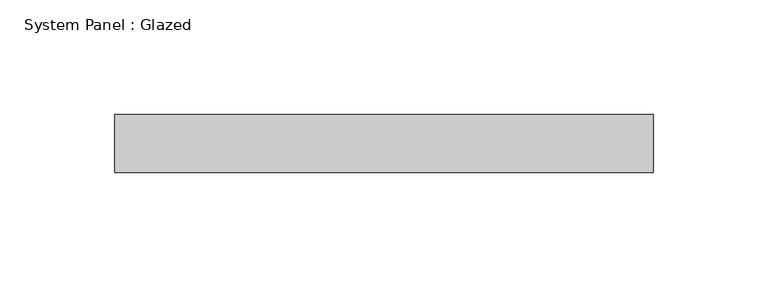
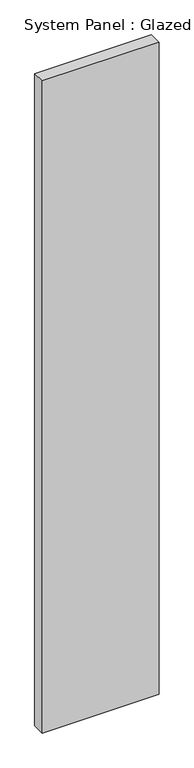
"""IFC4 building model written with IfcOpenShell, lengths in millimetres: plate geometry, System Panel : Glazed."""

from ifc_helpers import new_model, si_unit, origin, origin_with_axes, place, context, project, spatial, polyline, outline, extrude, source, transform, mapped, element, save


def system_panel_glazed_2f9bb5a6(model_context):
    return source(origin(), model_context, "Body", "SweptSolid", [
        extrude(outline(polyline([(117.475, 19.05), (-117.475, 19.05), (-117.475, 44.45), (117.475, 44.45), (117.475, 19.05)])), origin_with_axes(), (0.0, 0.0, 1.0), 1383.5980535),
    ])


if __name__ == "__main__":
    model = new_model("IFC4")
    model_context = context("Model", 3, world=origin())
    ifc_project = project(units=[si_unit("LENGTHUNIT", "METRE", prefix="MILLI")], contexts=[model_context])
    site = spatial("IfcSite", under=ifc_project)
    building = spatial("IfcBuilding", under=site)
    placement = place(None, origin())
    system_panel_glazed_shape = system_panel_glazed_2f9bb5a6(model_context)
    element("IfcPlate", 1, ObjectType="System Panel : Glazed", at=placement, inside=building, context=model_context, shape_type="MappedRepresentation", body=[
        mapped(system_panel_glazed_shape, transform((0.0, 0.0, 0.0), x_axis=(1.0, 0.0, 0.0), y_axis=(0.0, 1.0, 0.0), z_axis=(0.0, 0.0, 1.0))),
    ])
    save(model, "model.ifc")

# Revit data of these elements
# Type "System Panel : Glazed"
#   Construction Type Id = "GSP4R"
#   Analytic Construction = "1/8 in Pilkington single glazing"
#   Visual Light Transmittance = 0.9
#   Solar Heat Gain Coefficient = 0.86
#   Heat Transfer Coefficient (U) = 1.18115 BTU/(h·ft²·°F)
#   Define Thermal Properties by = 1
# Element 1 (IfcPlate, "System Panel : Glazed")
#   Materials on its faces: "Glass"
# Materials
#   "Glass": class "Glass", colour RGB 0 128 192, transparency 0.75, Description = "Soda Lime Glass", Cost = 0
